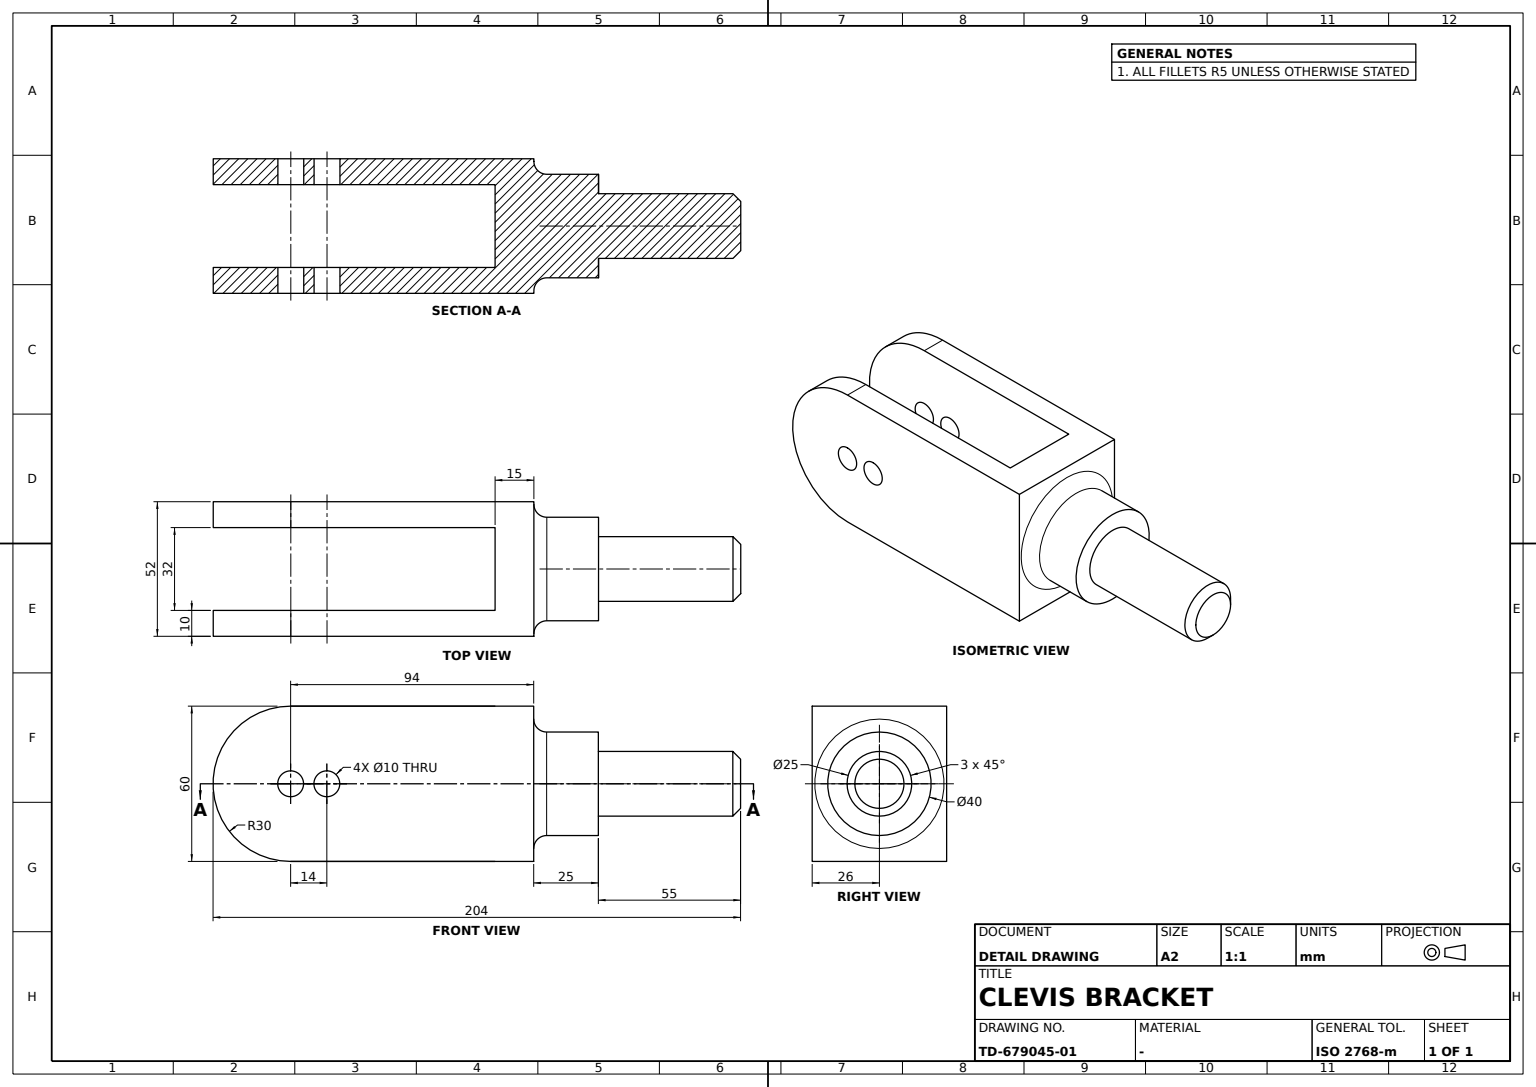
CATIA V5 part; units mm, degrees
sketch "Sketch1" plane through (0, 0, 0) normal (0, 1, 0) x (-1, 0, 0)
  line L0 (0, 30) -> (94, 30)
  point P0 (94, 0)
  line L1 (94, -30) -> (0, -30)
  point P1 (0, -30)
  arc A0 (94, -30) -> (94, 30) centre (94, 0) ccw
  point P2 (94, -30)
  line L2 (0, -30) -> (0, 30)
  circle A1 centre (94, 0) radius 5
  circle A2 centre (80, 0) radius 5
  dimension "length L0" = 94
  dimension "distance P1 y axis" = 0
  dimension "length L1" = 94
  dimension "radius A1" = 5
  dimension "radius A2" = 5
  constraint horizontal L0 x-axis
  constraint coincidence P0 x-axis
  constraint coincidence A0 P2
  constraint coincidence P2 L1
  constraint tangency A0 L1
  constraint vertical L2 y-axis
extrude "Pad1" add sketch "Sketch1" along normal blind 10
sketch "Sketch2" plane through (0, 10, 0) normal (0, 1, 0) x (-1, 0, 0)
  line L0 (0, 30) -> (15, 30)
  line L1 (15, 30) -> (15, -30)
  line L2 (15, -30) -> (0, -30)
  point P0 (0, -30)
  line L3 (0, -30) -> (0, 30)
  dimension "length L0" = 15
  dimension "length L1" = 60
  dimension "length L2" = 15
  constraint horizontal L0 x-axis
  constraint vertical L1 y-axis
  constraint vertical L3 y-axis
  constraint coincidence P0 y-axis
extrude "Pad2" add sketch "Sketch2" along normal blind 32
sketch "Sketch3" plane through (0, 42, 0) normal (0, 1, 0) x (-1, 0, 0)
  line L0 (0, 30) -> (94, 30)
  arc A0 (94, -30) -> (94, 30) centre (94, 0) ccw
  line L1 (94, -30) -> (0, -30)
  point P0 (0, -30)
  line L2 (0, 30) -> (0, -30)
  circle A1 centre (94, 0) radius 5
  circle A2 centre (80, 0) radius 5
  dimension "length L0" = 94
  dimension "radius A1" = 5
  dimension "radius A2" = 5
  constraint horizontal L0 x-axis
  constraint tangency A0 L0
  constraint tangency L1 A0
  constraint coincidence P0 y-axis
  constraint vertical L2 y-axis
extrude "Pad3" add sketch "Sketch3" along normal blind 10
sketch "Sketch4" plane through (0, 0, 0) normal (1, 0, 0) x (0, 1, 0)
  circle A0 centre (26, 0) radius 20
  dimension "radius A0" = 20
extrude "Pad4" add sketch "Sketch4" along normal blind 25
sketch "Sketch5" plane through (25, 0, 0) normal (1, 0, 0) x (0, 1, 0)
  circle A0 centre (26, 0) radius 12.5
  dimension "radius A0" = 12.5
extrude "Pad5" add sketch "Sketch5" along normal blind 55
chamfer "Chamfer1" distance 3 angle 45 1 edges at (80, 13.5, 0)
fillet "Fillet1" radius 5 1 edges at (0, 6, 0)
